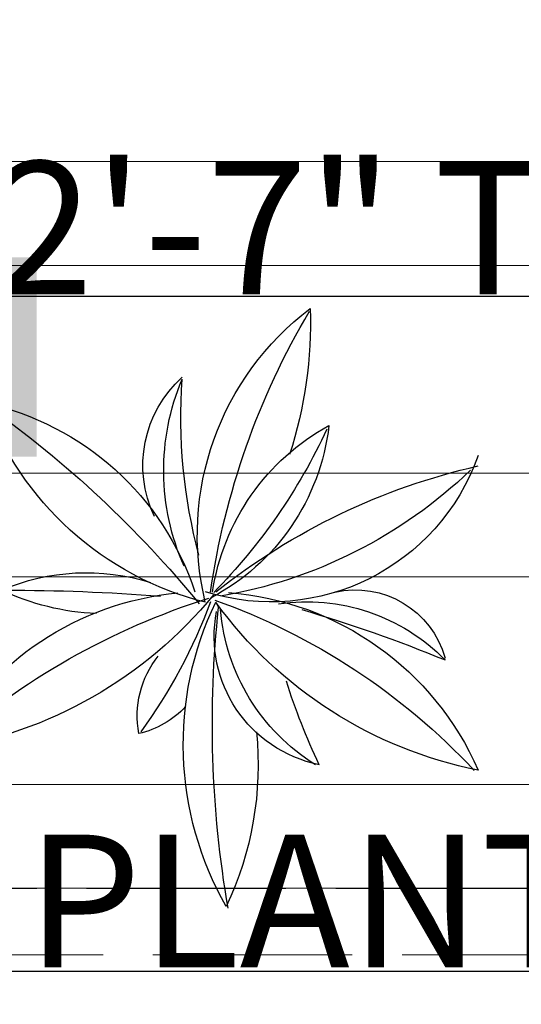
# Model space of a CAD drawing. Units: inches. Extents: x 351 to 1738, y -265 to 286.
# Tile 11 of 38: x 1112 to 1142, y -206 to -147. Entities that reach past the tile are written whole.
import ezdxf

# ---------------------------------------------------------------- set-up
doc = ezdxf.new("R2010")
doc.units = ezdxf.units.IN
doc.header["$MEASUREMENT"] = 0
doc.linetypes.add('ACAD_ISO02W100', pattern=[15, 12, -3])
for name, color, linetype, lineweight in [('A-ANNO-DIMS', 2, 'Continuous', 18), ('A-COLS-PATT', 6, 'Continuous', 13), ('A-FLOR-OVHD', 1, 'ACAD_ISO02W100', 18), ('A-FLOR-PATT', 9, 'Continuous', 9)]:
    doc.layers.add(name, color=color, linetype=linetype, lineweight=lineweight)
for name, color, linetype in [('CAY', 94, 'Continuous'), ('CHITIET', 144, 'Continuous'), ('netmanh', 9, 'Continuous'), ('VATDUNG', 9, 'Continuous')]:
    doc.layers.add(name, color=color, linetype=linetype)
doc.styles.get("Standard").update_dxf_attribs({"font": 'arial.ttf'})
doc.dimstyles.get("Standard").update_dxf_attribs({"dimtxt": 8, "dimasz": 5, "dimexe": 0.18, "dimexo": 0.0625, "dimgap": 0.09, "dimtad": 1, "dimtoh": 1, "dimzin": 0, "dimdsep": 46, "dimlunit": 4, "dimtxsty": 'Standard', "dimcen": 0, "dimclre": 256, "dimadec": 0, "dimazin": 0, "dimtfac": 1, "dimtofl": 0, "dimtmove": 0, "dimatfit": 3, "dimfxl": 1, "dimtolj": 1, "dimtzin": 0, "dimlwe": -1, "dimarcsym": 0})

# ---------------------------------------------------------------- blocks, each defined once
blk = doc.blocks.new('A$C5431134F')
at = {"layer": 'VATDUNG'}
for centre, radius, start, end in [((2160.8, 1662), 1245, 150.2411, 205.809), ((5177, 1582.5), 4150.3, 170.24, 186.1148), ((-65.9, 1738.8), 1267.2, 354.3326, 25.2804), ((1532.8, 1250.1), 499, 101.4267, 190.9877), ((193.1, 3473.3), 2507.8, 289.6318, 316.9416), ((2357.8, 162.2), 1629.1, 101.2486, 143.9899), ((1828.1, 1082.8), 773.2, 121.9055, 175.1859), ((1000.7, 2213.1), 1133.8, 274.4073, 336.4431), ((3715.1, 660.2), 2523.5, 154.6853, 162.4501), ((-246.7, 51.1), 1647.5, 39.15, 81.389), ((1000.7, 2213.1), 1133.8, 208.0484, 264.6491), ((1859.5, 3770.4), 2797.6, 228.5745, 252.3842), ((1101.5, 1552.5), 361.2, 169.1166, 218.9556), ((667.9, 1279.8), 349.9, 42.8374, 76.9786), ((-929.9, 388.9), 2082.1, 20.5138, 36.0242), ((1386.4, 1856.4), 738.5, 261.6389, 315.6255), ((-169.9, 6392.7), 5465.7, 286.3355, 292.415), ((1571.2, 1428.8), 356.3, 257.3557, 344.3532), ((624.5, 223.6), 940.4, 92.4374, 115.2956), ((-65.9, 1738.8), 1267.2, 330.7697, 331.9367), ((1294.4, -49.6), 1206.1, 104.1284, 160.1468), ((-2233.8, 3749.8), 4146.2, 305.4464, 320.7382), ((248.9, 8461.8), 7388, 269.91003, 274.50199), ((2052.7, 864.5), 1083.3, 166.3603, 232.9474), ((1250.8, 281.5), 836.9, 19.4342, 107.4357), ((625, 349.3), 851.8, 6.5073, 62.3609), ((754.1, -691.9), 1814.1, 46.1483, 80.3711), ((-70, 1420), 1084.7, 282.2423, 341.7321), ((546.4, 1826.6), 819.5, 246.7315, 287.3971), ((3885.3, 1488.7), 2894, 188.0959, 210.7226), ((1889.6, 1210.8), 871.9, 188.5552, 241.3289), ((-527.8, -458.7), 2192.5, 24.7599, 44.6473), ((2594.9, 3037.7), 2500, 231.5416, 257.1764), ((1738.9, 617.5), 897.6, 155.9893, 202.84), ((2946.5, 414), 2039.9, 165.0604, 184.0737), ((1214.1, 597.8), 452.1, 154.5276, 228.0163), ((-246.7, 51.1), 1647.5, 358.2222, 17.8583)]:
    blk.add_arc(centre, radius, start, end, dxfattribs=at)
blk = doc.blocks.new('A$C5A8625A6')
at = {"layer": 'CHITIET', "ltscale": 50, "xscale": -0.49, "yscale": 0.49, "zscale": 0.49, "rotation": 180}
blk.add_blockref('A$C5431134F', (0, 1120.2), dxfattribs=at)
blk = doc.blocks.new('A$C18571848')
at = {"layer": 'netmanh', "xscale": 0.5393606399999998, "yscale": 0.5393606399999998, "zscale": 0.5393606399999998}
blk.add_blockref('A$C5A8625A6', (0, 0), dxfattribs=at)
blk = doc.blocks.new('*D36')
at = {"layer": 'A-ANNO-DIMS', "transparency": 16777216}
for p, q in [((1073.569, -199.341), (1073.569, -204.202)), ((1105.198, -199.341), (1105.198, -204.202))]:
    blk.add_line(p, q, dxfattribs=at)
at = {"layer": 'A-ANNO-DIMS', "color": 0, "lineweight": -2, "transparency": 16777216}
for p, q in [((1078.569, -204.022), (1100.198, -204.022)), ((1105.198, -204.022), (1227.071, -204.022))]:
    blk.add_line(p, q, dxfattribs=at)
at = {"layer": 'A-ANNO-DIMS', "color": 0, "transparency": 16777216}
for points in [[(1078.569, -203.189), (1078.569, -204.856), (1073.569, -204.022)], [(1100.198, -203.189), (1100.198, -204.856), (1105.198, -204.022)]]:
    blk.add_solid(points, dxfattribs=at)
at = {"layer": 'Defpoints', "color": 0, "transparency": 16777216}
for p in [(1073.569, -199.278), (1105.198, -199.278), (1105.198, -204.022)]:
    blk.add_point(p, dxfattribs=at)
at = {"layer": 'A-ANNO-DIMS', "color": 0, "transparency": 16777216, "insert": (1168.634, -199.796), "char_height": 8, "attachment_point": 5}
blk.add_mtext('\\A1;PLANT A 2\'-7 1/2" TYP.', dxfattribs=at)
blk = doc.blocks.new('*D37')
at = {"layer": 'A-ANNO-DIMS', "color": 0, "lineweight": -2, "transparency": 16777216}
for p, q in [((1109.942, -168.369), (1109.942, -163.369)), ((1109.942, -163.369), (1158.933, -163.369)), ((1109.942, -194.278), (1109.942, -173.369))]:
    blk.add_line(p, q, dxfattribs=at)
at = {"layer": 'A-ANNO-DIMS', "transparency": 16777216}
for p, q in [((1105.26, -168.369), (1110.122, -168.369)), ((1105.26, -199.278), (1110.122, -199.278))]:
    blk.add_line(p, q, dxfattribs=at)
at = {"layer": 'A-ANNO-DIMS', "color": 0, "transparency": 16777216}
for points in [[(1109.109, -173.369), (1110.775, -173.369), (1109.942, -168.369)], [(1109.109, -194.278), (1110.775, -194.278), (1109.942, -199.278)]]:
    blk.add_solid(points, dxfattribs=at)
at = {"layer": 'Defpoints', "color": 0, "transparency": 16777216}
for p in [(1105.198, -168.369), (1109.942, -168.369), (1105.198, -199.278)]:
    blk.add_point(p, dxfattribs=at)
at = {"layer": 'A-ANNO-DIMS', "color": 0, "transparency": 16777216, "insert": (1134.482, -159.26), "char_height": 8, "attachment_point": 5}
blk.add_mtext('\\A1;2\'-7" TYP.', dxfattribs=at)

msp = doc.modelspace()

# ---------------------------------------------------------------- hatches: boundary and pattern name
at = {"layer": 'A-COLS-PATT'}
h = msp.add_hatch(color=256, dxfattribs=at)
h.dxf.hatch_style = 1
h.paths.add_polyline_path([(1112.704, 237.963), (1103.704, 237.963), (1103.704, 228.963), (1112.704, 228.963)])
h.paths.add_polyline_path([(1115.704, 237.963), (1112.704, 237.963), (1112.704, 228.963), (1115.704, 228.963)])
h.paths.add_polyline_path([(1043.704, 255.963), (1034.704, 255.963), (1034.704, 243.963), (1043.704, 243.963)])
h.paths.add_polyline_path([(1043.704, 210.963), (1034.704, 210.963), (1034.704, 198.963), (1043.704, 198.963)])
h.paths.add_polyline_path([(1043.704, -45.037), (1034.704, -45.037), (1034.704, -57.037), (1043.704, -57.037)])
h.paths.add_polyline_path([(1112.704, -45.037), (1103.704, -45.037), (1103.704, -57.037), (1112.704, -57.037)])
h.paths.add_polyline_path([(1112.704, -161.037), (1103.704, -161.037), (1103.704, -164.037), (1103.704, -173.037), (1112.704, -173.037)])
h.paths.add_polyline_path([(1043.704, -161.037), (1034.704, -161.037), (1034.704, -173.037), (1043.704, -173.037)])
h.paths.add_polyline_path([(1248.549, -164.037), (1236.549, -164.037), (1236.549, -173.037), (1248.549, -173.037)])
h.paths.add_polyline_path([(1248.549, -50), (1236.549, -50), (1236.549, -59), (1248.549, -59)])
h.paths.add_polyline_path([(1248.704, 73.463), (1244.704, 73.463), (1244.704, 64.463), (1248.704, 64.463)])
h.paths.add_polyline_path([(1244.704, 73.463), (1236.704, 73.463), (1236.704, 64.463), (1244.704, 64.463)])
h.paths.add_polyline_path([(1248.704, 237.963), (1236.704, 237.963), (1236.704, 228.963), (1248.704, 228.963)])
h.paths.add_polyline_path([(1392.204, 237.963), (1380.204, 237.963), (1380.204, 228.963), (1392.204, 228.963)])
h.paths.add_polyline_path([(1536.064, 237.963), (1524.064, 237.963), (1524.064, 228.963), (1536.064, 228.963)])
h.paths.add_polyline_path([(1536.064, 73.463), (1524.064, 73.463), (1524.064, 64.463), (1536.064, 64.463)])
h.paths.add_polyline_path([(1384.204, 73.463), (1380.204, 73.463), (1380.204, 64.463), (1384.204, 64.463)])
h.paths.add_polyline_path([(1392.064, 73.463), (1384.204, 73.463), (1384.204, 64.463), (1392.064, 64.463)])
h.paths.add_polyline_path([(1536.064, -53.037), (1524.064, -53.037), (1524.064, -57.037), (1536.064, -57.037)])
h.paths.add_polyline_path([(1536.064, -48.037), (1524.064, -48.037), (1524.064, -53.037), (1536.064, -53.037)])
h.paths.add_polyline_path([(1392.064, -48.037), (1380.064, -48.037), (1380.064, -56.5), (1380.065, -57.037), (1392.064, -57.037)])
h.paths.add_polyline_path([(1536.064, -164.037), (1524.064, -164.037), (1524.064, -173.037), (1536.064, -173.037)])
at = {"layer": 'A-FLOR-PATT', "transparency": 33554559}
h = msp.add_hatch(dxfattribs=at)
h.set_pattern_fill('ANSI37', color=256, scale=200, angle=135)
h.set_pattern_definition([(180, (1112.704, -164.037), (-2e-15, -25), []), (270, (1112.704, -164.037), (25, -5e-15), [])])
h.paths.add_polyline_path([(1380.064, 73.463), (1380.132, 148.463), (1338.064, 148.463), (1290.704, 148.463), (1290.704, 88.463), (1248.704, 88.463), (1248.704, -2.009), (1244.704, -2.009), (1244.704, 142.457), (1160.704, 142.457), (1160.704, 158.963), (1160.704, 170.137), (1160.704, 206.137), (1160.704, 228.963), (1112.704, 228.963), (1112.704, 209.963), (1112.704, 168.963), (1124.704, 168.963), (1124.704, 162.963), (1112.704, 162.963), (1112.704, 64.463), (1112.704, 60.463), (1112.704, 0.463), (1112.704, -48.026), (1146.804, -47.981), (1146.804, -35.691), (1207.804, -35.691), (1207.804, -47.902), (1236.542, -47.864), (1236.544, -50.009), (1248.5, -50.009), (1248.506, -102.915), (1248.512, -150.915), (1248.514, -164.037), (1248.549, -164.037), (1273.017, -164.037), (1273.017, -128.799), (1355.24, -128.799), (1355.24, -164.037), (1384.204, -164.037), (1384.204, -57.037), (1380.064, -57.037), (1380.064, -48.037), (1392.064, -48.037), (1392.064, -53.037), (1406.549, -53.037), (1406.549, -57.037), (1401.204, -57.037), (1401.204, -147.037), (1468.204, -147.037), (1468.204, -138.5), (1472.204, -138.5), (1472.204, -102.5), (1468.204, -102.5), (1468.204, -57.037), (1442.549, -57.037), (1442.549, -53.037), (1463.049, -53.037), (1463.049, -40.747), (1524.049, -40.747), (1524.049, -48.037), (1536.064, -48.037), (1536.064, -53.037), (1557.704, -53.037), (1557.704, 204.963), (1384.204, 204.963), (1384.204, 73.463), (1392.064, 73.463), (1392.064, 64.463), (1384.204, 64.463), (1384.204, -3.5), (1380.204, -3.537), (1380.204, 64.463), (1380.064, 64.463)])
h.paths.add_polyline_path([(1510.714, 86.458, -0.103984), (1511.661, 85.595, 0.470438), (1510.158, 87.614, 0.0961)], flags=16)
h.paths.add_polyline_path([(1510.443, 100.266, 0.009798), (1504.693, 100.48, 0.02879), (1504.6, 99.767, -0.165331), (1505.519, 96.135, -0.143601)], flags=16)
h.paths.add_polyline_path([(1487.201, 85.595, -0.103984), (1488.148, 86.458, 0.0961), (1488.704, 87.614, 0.470438)], flags=0)
h.paths.add_polyline_path([(1495.052, 100.43), (1494.178, 100.43, -0.026463), (1494.262, 99.774, -0.144219)], flags=16)
h.paths.add_polyline_path([(1444.485, 86.458, -0.103984), (1445.433, 85.595, 0.470438), (1443.93, 87.614, 0.0961)], flags=16)
h.paths.add_polyline_path([(1420.972, 85.595, -0.103984), (1421.92, 86.458, 0.0961), (1422.475, 87.614, 0.470438)], flags=16)
h.paths.add_polyline_path([(1428.632, 100.335, 0.001054), (1427.971, 100.309, -0.021524), (1428.033, 99.774, -0.114301)], flags=16)
h.paths.add_polyline_path([(1419.906, 143.708, 0.024979), (1420.222, 157.526), (1421.573, 159.101), (1421.573, 175.369), (1391.393, 175.369), (1391.393, 200.519), (1542.294, 200.519), (1542.294, 175.369), (1512.028, 175.369, 0.019865), (1511.521, 153.838, 0.025134), (1512.758, 118.323, 0.020553), (1512.942, 115.253), (1419.834, 115.253, -0.000414), (1419.843, 124.798), (1413.059, 124.798), (1413.059, 84.437, -0.061853), (1415.831, 80.45, -0.093077), (1420.972, 85.595, -0.267537), (1422.371, 84.732, 0.08511), (1424.052, 84.616, -0.885393), (1424.033, 84.851, -1.125815), (1424.073, 84.366, -0.087987), (1422.371, 84.732, -0.267537), (1422.326, 83.089, -0.370542), (1420.972, 85.595, 0.093077), (1415.831, 80.45, -0.087414), (1417.914, 73.937), (1418.941, 73.937, 0.02725), (1418.913, 76.906, -0.115703), (1421.051, 73.937), (1445.354, 73.937, -0.115703), (1447.492, 76.906, 0.02725), (1447.464, 73.937), (1448.491, 73.937, -0.087414), (1450.574, 80.45, 0.093077), (1445.433, 85.595, -0.370542), (1444.079, 83.089, -0.267537), (1444.034, 84.732, -0.087987), (1442.332, 84.366, -1.125815), (1442.372, 84.851, -2.032736), (1442.364, 84.368, 0.086378), (1444.034, 84.732, -0.267537), (1445.433, 85.595, -0.093077), (1450.574, 80.45, -0.257732), (1466.483, 90.927, -0.47867), (1468.832, 91.907, -0.47867), (1471.18, 90.927, -0.26264), (1483.053, 81.78, -0.071866), (1487.201, 85.595, -0.267537), (1488.6, 84.732, 0.08511), (1490.28, 84.616, -0.885393), (1490.262, 84.851, -1.125815), (1490.301, 84.366, -0.087987), (1488.6, 84.732, -0.267537), (1488.554, 83.089, -0.370542), (1487.201, 85.595, 0.071866), (1483.053, 81.78, -0.132065), (1484.143, 73.937), (1485.169, 73.937, 0.02725), (1485.142, 76.906, -0.115703), (1487.28, 73.937), (1511.582, 73.937, -0.115703), (1513.72, 76.906, 0.02725), (1513.693, 73.937), (1514.719, 73.937, -0.087414), (1516.802, 80.45, 0.093077), (1511.661, 85.595, -0.370542), (1510.308, 83.089, -0.267537), (1510.262, 84.732, -0.087987), (1508.561, 84.366, -1.125815), (1508.601, 84.851, -2.032736), (1508.592, 84.368, 0.086378), (1510.262, 84.732, -0.267537), (1511.661, 85.595, -0.093077), (1516.802, 80.45, -0.061853), (1519.575, 84.437), (1519.575, 73.937), (1413.059, 73.937), (1413.059, 124.798), (1419.843, 124.798, -0.000821)], flags=16)
h.paths.add_polyline_path([(1220.149, 54.133, -0.103984), (1220.869, 53.476, 0.470438), (1219.727, 55.011, 0.0961)], flags=16)
h.paths.add_polyline_path([(1219.944, 64.626, 0.009798), (1215.574, 64.789, 0.02879), (1215.503, 64.247, -0.165331), (1216.201, 61.487, -0.143601)], flags=16)
h.paths.add_polyline_path([(1209.779, 64.449, 0.097446), (1209.339, 64.751), (1208.247, 64.751, 0.12739), (1207.7, 64.326, 0.171586), (1206.95, 61.475, -0.158854), (1207.636, 59.45, 0.015898), (1207.795, 59.218, 0.061546), (1208.598, 59.616, 0.175416), (1208.638, 60.099, -0.284779), (1209.348, 62.472, 0.326216)], flags=16)
h.paths.add_polyline_path([(1169.818, 54.133, -0.103984), (1170.538, 53.476, 0.470438), (1169.396, 55.011, 0.0961)], flags=16)
h.paths.add_polyline_path([(1159.017, 62.472, 0.284764), (1158.307, 60.099, -0.175433), (1158.267, 59.616, 0.39293), (1159.448, 64.449, -0.32623)], flags=16)
h.paths.add_polyline_path([(1156.342, 58.239, -0.178321), (1154.011, 55.31, -0.174736), (1154.722, 55.233, -0.200802), (1156.27, 56.086, 0.12699), (1157.283, 58.991, -0.091205)], flags=16)
h.paths.add_polyline_path([(1156.624, 61.413, 0.157275), (1157.316, 64.247, 0.169622)], flags=16)
h.paths.add_polyline_path([(1152.67, 54.133, -0.0961), (1151.95, 53.476, 0.064076), (1154.465, 54.384, 0.199016)], flags=16)
h.paths.add_polyline_path([(1202.281, 53.476, -0.103984), (1203, 54.133, 0.0961), (1203.423, 55.011, 0.470438)], flags=0)
h.paths.add_polyline_path([(1151.139, 97.64, 0.024979), (1151.379, 108.141), (1152.406, 109.338), (1152.406, 121.701), (1129.47, 121.701), (1129.47, 140.814), (1244.149, 140.814), (1244.149, 121.701), (1221.148, 121.701, 0.019865), (1220.763, 105.338, 0.025134), (1221.703, 78.349, 0.020553), (1221.843, 76.016), (1151.078, 76.016, -0.128743), (1148.786, 65.037, 0.539352), (1150.327, 64.171, -0.027594), (1163.481, 64.751, 0.097695), (1163.04, 64.449, 0.326216), (1163.471, 62.472, -0.284777), (1164.181, 60.099, -0.194757), (1165.846, 61.443, -0.155402), (1165.172, 64.247, -0.166022), (1165.869, 61.475, -0.177014), (1167.852, 62.77, -0.448203), (1169.974, 60.807, -0.393499), (1167.679, 57.86, -0.895548), (1168.438, 54.524, -0.355767), (1166.218, 56.086, -0.066024), (1165.505, 57.539), (1165.251, 56.243, -0.371732), (1164.02, 59.758, -0.373614), (1163.04, 64.449, -0.097695), (1163.481, 64.751, 0.021354), (1153.294, 64.429, -0.134183), (1156.695, 61.368, 0.186873), (1154.636, 62.77, 0.448203), (1152.514, 60.807, 0.403726), (1154.905, 57.846, 0.711219), (1153.334, 55, 0.53154), (1151.95, 53.476, -0.267537), (1153.013, 52.821, 0.08511), (1154.29, 52.732, -0.885393), (1154.276, 52.911, -1.125815), (1154.306, 52.543, -0.087987), (1153.013, 52.821, -0.267537), (1152.978, 51.572, -0.370542), (1151.95, 53.476, 0.093077), (1148.043, 49.566, -0.087414), (1149.626, 44.617), (1150.406, 44.617, 0.02725), (1150.385, 46.873, -0.115703), (1152.01, 44.617), (1170.478, 44.617, -0.115703), (1172.103, 46.873, 0.02725), (1172.082, 44.617), (1172.862, 44.617, -0.087414), (1174.445, 49.566, 0.093077), (1170.538, 53.476, -0.370542), (1169.51, 51.572, -0.267537), (1169.475, 52.821, -0.087987), (1168.182, 52.543, -1.125815), (1168.212, 52.911, -2.032736), (1168.206, 52.544, 0.086378), (1169.475, 52.821, -0.267537), (1170.538, 53.476, -0.093077), (1174.445, 49.566, -0.257732), (1186.536, 57.528, -0.47867), (1188.321, 58.273, -0.47867), (1190.106, 57.528, -0.26264), (1199.128, 50.577, -0.071866), (1202.281, 53.476, -0.267537), (1203.344, 52.821, 0.08511), (1204.621, 52.732, -0.885393), (1204.607, 52.911, -1.125815), (1204.637, 52.543, -0.087987), (1203.344, 52.821, -0.267537), (1203.309, 51.572, -0.370542), (1202.281, 53.476, 0.071866), (1199.128, 50.577, -0.132065), (1199.957, 44.617), (1200.737, 44.617, 0.02725), (1200.716, 46.873, -0.115703), (1202.341, 44.617), (1220.809, 44.617, -0.115703), (1222.434, 46.873, 0.02725), (1222.413, 44.617), (1223.193, 44.617, -0.087414), (1224.776, 49.566, 0.093077), (1220.869, 53.476, -0.370542), (1219.841, 51.572, -0.267537), (1219.806, 52.821, -0.087987), (1218.513, 52.543, -1.125815), (1218.543, 52.911, -2.032736), (1218.537, 52.544, 0.086378), (1219.806, 52.821, -0.267537), (1220.869, 53.476, -0.093077), (1224.776, 49.566, -0.061853), (1226.883, 52.597), (1226.883, 44.617), (1145.936, 44.617), (1145.936, 83.269), (1151.091, 83.269, -0.000821)], flags=16)
h.paths.add_polyline_path([(1218.01, 57.86, -0.895548), (1218.769, 54.524, -0.355767), (1216.549, 56.086, -0.066024), (1215.836, 57.539), (1215.582, 56.243, -0.371732), (1214.351, 59.758, -0.373614), (1213.371, 64.449, 0.326216), (1213.802, 62.472, -0.284777), (1214.512, 60.099, -0.194757), (1216.177, 61.443, -0.179991), (1218.183, 62.77, -0.448203), (1220.305, 60.807, -0.393499)], flags=16)
h.paths.add_polyline_path([(1424.735, 91.363, -0.393499), (1421.715, 95.241, -0.448203), (1424.507, 97.824, -0.179991), (1427.147, 96.077, -0.194757), (1429.338, 94.309, -0.284777), (1430.272, 97.432, 0.326216), (1430.839, 100.034, -0.373614), (1429.55, 93.861, -0.371732), (1427.929, 89.235), (1427.596, 90.941, -0.066024), (1426.657, 89.029, -0.355767), (1423.736, 86.973, -0.895548)], flags=16)
h.paths.add_polyline_path([(1238.033, 131.257, -1), (1227.329, 131.257, -1)], flags=0)
h.paths.add_polyline_path([(1235.357, 131.257, -1), (1230.005, 131.257, -1)], flags=0)
h.paths.add_polyline_path([(1214.039, 54.243, 0.154382), (1214.38, 53.992, 0.358955), (1213.613, 54.016, 0.603948), (1214.379, 53.657, 0.371319), (1213.968, 52.872, 0.187994), (1214.312, 52.809, -0.592455), (1213.953, 52.967, -0.294279), (1214.083, 53.691, -1.300187), (1213.881, 54.134, -0.283762), (1214.469, 53.896, 1.15094)], flags=16)
h.paths.add_polyline_path([(1212.091, 56.286, -0.408434), (1211.337, 56.445, -0.036259), (1211.098, 56.848, -0.236098), (1211.59, 56.63, 0.035345), (1211.835, 56.543, -0.475241), (1212.091, 56.286, -0.475241), (1212.438, 56.182, 0.035345), (1212.631, 56.007, -0.236098), (1213.056, 55.676, -0.036259), (1212.588, 55.697, -0.408434)], flags=16)
h.paths.add_polyline_path([(1211.469, 50.297, 0.296043), (1210.47, 50.527, 0.310883), (1211.931, 50.148, 0.021255)], flags=16)
h.paths.add_polyline_path([(1213.739, 51.818, -0.036259), (1213.271, 51.838, -0.408434), (1212.774, 52.427, -0.094786), (1212.293, 50.703, 1.150474), (1212.911, 50.232, 0.166288), (1213.265, 50.68, -0.025254), (1212.603, 50.13, 1.087932), (1212.471, 49.407, 0.166288), (1213.02, 49.251, -0.016128), (1212.567, 49.563, -0.286859), (1212.217, 49.638, 0.022156), (1212.046, 50.055, -0.64613), (1212.185, 50.498, 0.088412), (1212.732, 52.077, -1.186037), (1213.121, 52.323, 0.035345), (1213.314, 52.148, -0.236098)], flags=16)
h.paths.add_polyline_path([(1212.094, 50.342, -0.048524), (1211.54, 49.605, -1.103834), (1211.397, 48.738, -0.785515), (1211.683, 48.254, -0.392043), (1210.948, 48.525, -0.392819), (1210.561, 47.995, -0.592455), (1210.201, 48.153, -0.294279), (1210.331, 48.877, -0.704172), (1210.316, 49.592, -0.679344), (1210.729, 50.112, 0.563676)], flags=16)
h.paths.add_polyline_path([(1211.274, 49.829, -0.139826), (1210.745, 49.859, -0.217879), (1210.948, 49.509, -0.498572)], flags=0)
h.paths.add_polyline_path([(1433.426, 81.49, -0.181571), (1434.245, 81.788, -0.008067), (1433.726, 82.205, 0.045578), (1432.755, 81.242, 0.179011)], flags=16)
h.paths.add_polyline_path([(1434.146, 81.009, -0.132442), (1433.645, 80.771, 0.259089), (1433.234, 80.471, -0.180211), (1433.392, 80.805, -0.16994), (1432.758, 81.109, 0.032652), (1433.273, 80.474, -0.493363), (1434.046, 80.146, -0.390497)], flags=16)
h.paths.add_polyline_path([(1434.83, 80.047, -0.947538), (1435.294, 79.576, -0.299128), (1434.625, 79.404, -0.270439), (1435.01, 78.591, -0.592455), (1434.537, 78.382, -0.392819), (1434.027, 79.08, -0.392043), (1433.06, 78.723, -0.352042), (1433.003, 79.197, -0.197216), (1433.75, 79.734, -0.71364), (1434.447, 79.939, -0.21479), (1434.819, 80.475, 0.408833), (1435.075, 80.803, -0.226152)], flags=16)
h.paths.add_polyline_path([(1432.67, 81.217, -0.454218), (1431.897, 79.923, -0.414411), (1431.301, 80.035, 0.016129), (1431.897, 80.445, 0.27957), (1432.073, 80.871, -0.289504), (1431.103, 81.321, -0.414411), (1430.978, 81.915, 0.01613), (1431.586, 81.521, 0.341293), (1432.125, 81.583, -0.813186)], flags=16)
h.paths.add_polyline_path([(1429.893, 86.381, -0.947538), (1430.358, 85.91, -0.173106), (1429.984, 85.712, -0.038817), (1431.625, 84.214, -0.0879), (1432.097, 88.549, -0.049768), (1431.254, 88.49, -0.236098), (1431.814, 88.925, 0.035345), (1432.067, 89.155, -0.475241), (1432.524, 89.291, -0.475241), (1432.86, 89.63, 0.035345), (1433.182, 89.744, -0.236098), (1433.83, 90.032, -0.036259), (1433.516, 89.502, -0.408434), (1432.524, 89.291, -0.312424), (1432.106, 88.58, 0.088559), (1431.625, 84.214, -0.408434), (1430.971, 83.439, -0.036259), (1430.355, 83.412, -0.236098), (1430.914, 83.847, 0.035345), (1431.168, 84.078, -0.475241), (1431.625, 84.214, 0.038817), (1429.984, 85.712, -0.321732), (1429.333, 86.048, -0.32743), (1429.883, 86.809, 0.408833), (1430.138, 87.138, -0.226152)], flags=16)
h.paths.add_polyline_path([(1211.206, 58.616, -0.999784), (1211.336, 59.323, -0.614994)], flags=16)
h.paths.add_polyline_path([(1210.288, 49.429, 0.154382), (1210.629, 49.178, 0.358955), (1209.861, 49.202, 0.603948), (1210.627, 48.843, -0.534825), (1210.806, 49.295, 0.748346)], flags=16)
h.paths.add_polyline_path([(1209.589, 51.828, -0.008791), (1209.775, 51.753, 0.112231), (1209.466, 52.019, 1.418851), (1209.014, 51.708, -0.458726), (1208.651, 51.073, -0.592455), (1208.291, 51.232, -0.294279), (1208.421, 51.955, -1.300187), (1208.219, 52.398, -0.226005), (1208.719, 52.257, -0.475519), (1209.158, 52.369, -1.455499), (1209.603, 52.664, 0.421305), (1209.191, 52.262, -0.591212), (1208.979, 51.796, 0.497399), (1209.773, 51.333, 0.649312)], flags=16)
h.paths.add_polyline_path([(1208.029, 52.041, 0.544667), (1208.832, 52.045, 0.220132)], flags=0)
h.paths.add_polyline_path([(1210.438, 51.425, -0.2042), (1210.277, 52.018, 0.270826), (1209.915, 52.897, 0.324115)], flags=0)
h.paths.add_polyline_path([(1209.668, 52.407, -0.60139), (1208.99, 52.221, -0.394916), (1208.248, 52.83, -0.836792), (1208.651, 53.017, -0.338488), (1209.039, 52.571, 0.194138), (1209.191, 52.262, 0.413995), (1209.712, 52.475, 0.51771), (1210.503, 51.416, 0.401922), (1209.493, 50.93, 0.206396), (1209.516, 50.165, -0.319463), (1210.417, 51.418, -0.466635)], flags=16)
h.paths.add_polyline_path([(1206.601, 56.086, -0.355767), (1204.381, 54.524, -0.921198), (1205.236, 57.846, 0.206569), (1207.614, 58.991, -0.12699)], flags=16)
h.paths.add_polyline_path([(1435.487, 82.816, 0.527765), (1436.615, 83.361, 0.50854), (1437.05, 82.433, 0.592455), (1437.524, 82.641, 0.331245), (1436.963, 83.548, 0.387863), (1437.808, 83.626, 0.592954), (1437.618, 84.176, 0.226016), (1436.961, 83.99, 0.318205), (1437.588, 84.854, 0.689374), (1437.05, 84.991, 0.335765), (1436.539, 84.41, -0.156993), (1436.404, 84.065, -0.434611), (1436.961, 83.99, -0.21479), (1437.333, 84.526, 0.408833), (1437.588, 84.854, -0.226152), (1437.343, 84.097, -0.947538), (1437.808, 83.626, -0.299128), (1437.139, 83.455, -0.270439), (1437.524, 82.641, -0.592455), (1437.05, 82.433, -0.392819), (1436.541, 83.13, -0.43966), (1435.475, 82.794, -0.174614), (1435.942, 82.244, -0.206396), (1435.912, 81.237, -0.270826), (1435.125, 82.208, 0.207976), (1434.686, 82.904, -0.196495)], flags=16)
h.paths.add_polyline_path([(1435.386, 84.832, 0.270811), (1434.91, 83.676, -0.204217), (1434.699, 82.895, 0.324115)], flags=0)
h.paths.add_polyline_path([(1435.68, 84.18, -0.217656), (1435.554, 83.304, -0.176705), (1436.236, 83.778, -0.373036)], flags=0)
h.paths.add_polyline_path([(1435.566, 100.034, 0.326216), (1436.133, 97.432, -0.284777), (1437.067, 94.309, -0.194757), (1439.258, 96.077, -0.155402), (1438.371, 99.767, -0.166022), (1439.289, 96.12, -0.177014), (1441.897, 97.824, -0.448203), (1444.69, 95.241, -0.393499), (1441.67, 91.363, -0.895548), (1442.669, 86.973, -0.355767), (1439.748, 89.029, -0.066024), (1438.809, 90.941), (1438.476, 89.235, -0.371732), (1436.855, 93.861, -0.373614)], flags=16)
h.paths.add_polyline_path([(1191.252, 49.507, -0.274022), (1190.658, 48.409, 0.267537), (1191.311, 47.344, 0.370542)], flags=0)
h.paths.add_polyline_path([(1190.301, 49.717, 0.199016), (1188.619, 49.04, 0.064076), (1191.252, 49.507, -0.0961)], flags=0)
h.paths.add_polyline_path([(1189.518, 47.857, 1.125815), (1189.676, 47.523, 2.044605)], flags=0)
h.paths.add_polyline_path([(1464.974, 80.372, 0.274022), (1465.756, 78.927, -0.083013)], flags=0)
h.paths.add_polyline_path([(1464.974, 80.372, 0.370542), (1464.897, 77.525, 0.576324)], flags=0)
h.paths.add_polyline_path([(1464.974, 80.372, -0.470438), (1467.284, 81.372, -0.0961), (1466.226, 80.648, -0.199016), (1468.439, 79.757, -0.064076)], flags=0)
h.paths.add_polyline_path([(1189.511, 56.43, -0.259467), (1188.321, 56.391, -0.259467), (1187.13, 56.43, 0.08511), (1188.193, 55.716, -0.885393), (1188.27, 55.878, -1.196013), (1188.355, 55.442, 0.101459)], flags=0)
h.paths.add_polyline_path([(1188.321, 57.596, 0.078072), (1187.678, 57.24, 0.01555), (1188.321, 57.136, 0.01555), (1188.964, 57.24, 0.078072)], flags=0)
h.paths.add_polyline_path([(1190.164, 55.365, -0.576324), (1190.106, 57.528, -0.198294), (1188.321, 58.319, -0.198294), (1186.536, 57.528, -0.576324), (1186.477, 55.365, -0.370542), (1186.536, 57.528, 0.198294), (1188.321, 58.319, 0.198294), (1190.106, 57.528, -0.370542)], flags=0)
h.paths.add_polyline_path([(1188.372, 55.878, 1.125814), (1188.529, 55.544, 2.044605)], flags=0)
h.paths.add_polyline_path([(1186.341, 49.717, -0.0961), (1185.389, 49.507, 0.064076), (1188.022, 49.04, 0.199016)], flags=0)
h.paths.add_polyline_path([(1185.389, 49.507, -0.267537), (1185.984, 48.409, 0.08511), (1187.046, 47.695, -0.885393), (1187.123, 47.857, -1.125815), (1186.966, 47.523, -0.087987), (1185.984, 48.409, -0.267537), (1185.331, 47.344, -0.370542)], flags=0)
h.paths.add_polyline_path([(1399.441, 187.944, -1), (1413.525, 187.944, -1)], flags=0)
h.paths.add_polyline_path([(1402.962, 187.944, -1), (1410.004, 187.944, -1)], flags=0)
h.paths.add_polyline_path([(1357.663, -72.245), (1377.272, -72.245), (1377.272, -91.854), (1357.663, -91.854)], flags=16)
h.paths.add_polyline_path([(1467.256, 78.201, -1.125815), (1467.049, 77.761, -2.044605)], flags=0)
h.paths.add_polyline_path([(1468.822, 88.714, 0.941125), (1469.106, 88.316, 1.137152), (1468.765, 88.755, 0.890986), (1468.99, 88.245, 0.094828), (1470.398, 89.481, -0.267537), (1471.18, 90.927, -0.028123), (1469.678, 90.547, -0.028774), (1469.948, 90.311, -0.020327), (1468.832, 90.41, -0.020327), (1467.716, 90.311, -0.028774), (1467.986, 90.547, -0.028123), (1466.483, 90.927, -0.267537), (1467.265, 89.481, 0.08511), (1468.663, 88.542, -1.202316)], flags=0)
h.paths.add_polyline_path([(1178.25, 124.523, -0.119929), (1165.65, 124.145, -0.107349), (1159.133, 124.446, -0.102891), (1159.132, 130.465, -0.074897), (1158.993, 137.956, 0.002027), (1167.844, 137.479, -0.07553), (1180.337, 137.666, -0.075861), (1186.502, 137.688, -0.14099), (1186.272, 130.046, -0.095481), (1186.729, 124.748, -0.10603)], flags=0)
h.paths.add_polyline_path([(1469.225, 79.757, -0.199016), (1471.437, 80.648, -0.0961), (1470.379, 81.372, -0.470438), (1472.689, 80.372, -0.370542), (1472.766, 77.525, -0.267537), (1471.907, 78.927, -0.087986), (1470.615, 77.761, -1.125849), (1470.408, 78.201, -2.032736), (1470.642, 77.778, 0.086378), (1471.907, 78.927, -0.267537), (1472.689, 80.372, -0.064076)], flags=0)
h.paths.add_polyline_path([(1430.423, 186.902, -0.074897), (1430.24, 196.758, 0.002027), (1441.887, 196.131, -0.07553), (1458.326, 196.377, -0.075861), (1466.438, 196.406, -0.14099), (1466.136, 186.35, -0.095481), (1466.737, 179.378, -0.10603), (1455.58, 179.082, -0.119929), (1439, 178.585, -0.107349), (1430.425, 178.981, -0.102891)], flags=0)
h.paths.add_polyline_path([(1162.258, 49.939, 0.335765), (1161.87, 49.497, -0.156994), (1161.767, 49.235, -0.434611), (1162.19, 49.178, -0.21479), (1162.473, 49.585, 1.529195)], flags=16)
h.paths.add_polyline_path([(1161.683, 49.021, 0.581518), (1161.268, 49.583, 0.592761)], flags=16)
h.paths.add_polyline_path([(1162.602, 48.058, 0.371319), (1162.192, 48.843, 0.434533), (1162.88, 48.962, 0.185081), (1162.197, 48.926, 1.121837)], flags=16)
h.paths.add_polyline_path([(1161.443, 48.941, -1.307104), (1161.495, 48.571, -0.217752), (1161.136, 48.254, 0.697303), (1161.871, 49.048, 0.121514)], flags=16)
h.paths.add_polyline_path([(1162.531, 49.429, -0.207084), (1162.05, 49.146, -0.99203)], flags=16)
h.paths.add_polyline_path([(1161.304, 49.578, -0.719667), (1161.513, 50.079, -0.130428), (1160.836, 50.168, 0.039593)], flags=0)
h.paths.add_polyline_path([(1162.036, 50.584, -0.008067), (1161.642, 50.9, 0.029367), (1161.35, 50.297, -0.205788)], flags=16)
h.paths.add_polyline_path([(1162.882, 51.392, -0.124733), (1162.763, 51.828, -0.101191), (1162.399, 51.438, -0.153425)], flags=0)
h.paths.add_polyline_path([(1164.235, 51.85, -0.309107), (1164.513, 51.136, -0.627125), (1163.781, 51.603, -0.685909), (1162.777, 51.219, -0.233285), (1163.303, 50.165, -0.270826), (1162.705, 50.903, 0.2042), (1162.381, 51.425, 0.204182), (1162.542, 52.018, -0.270841), (1162.903, 52.897, -0.127261), (1163.219, 52.529, -1.168681), (1163.781, 52.587, -0.329112), (1164.168, 53.017, -0.836792), (1164.571, 52.83, -0.193341), (1164.391, 52.338, -0.947538), (1164.744, 51.981, -0.299128)], flags=16)
h.paths.add_polyline_path([(1163.598, 51.937, -1.262956), (1163.236, 51.831, 0.012575), (1162.971, 51.721, 0.230657), (1163.151, 52.407, -0.164898), (1163.178, 52.661, -0.44932), (1163.628, 52.262, -0.721477), (1164.154, 52.088, -0.849998)], flags=0)
h.paths.add_polyline_path([(1161.613, 58.616, -0.980413), (1161.525, 59.049, -2.908935)], flags=16)
h.paths.add_polyline_path([(1160.252, 49.166, -0.414411), (1159.799, 49.251, 0.016129), (1160.252, 49.563, 0.27957), (1160.386, 49.887, -0.289504), (1159.649, 50.229, -0.414411), (1159.554, 50.68, 0.01613), (1160.015, 50.381, 0.617885), (1160.526, 50.703, -0.094786), (1160.045, 52.427, -0.140444), (1159.682, 52.042, -0.057856), (1159.3, 51.872, 0.544843), (1160.046, 52.419, -0.088122), (1160.404, 55.721, -0.049768), (1159.763, 55.676, -0.236098), (1160.188, 56.007, 0.035345), (1160.381, 56.182, -0.475241), (1160.728, 56.286, -0.475241), (1160.984, 56.543, 0.035345), (1161.229, 56.63, -0.236098), (1161.721, 56.848, -0.036259), (1161.482, 56.445, -0.408434), (1160.728, 56.286, -0.312424), (1160.411, 55.745, 0.088559), (1160.045, 52.427, 0.107081), (1160.634, 50.498, -0.494798), (1160.839, 50.149, -0.454218)], flags=16)
h.paths.add_polyline_path([(1160.666, 49.808, -2.076528), (1160.828, 50.172, 0.019586)], flags=0)
h.paths.add_polyline_path([(1158.439, 53.992, 0.154382), (1158.78, 54.243, 0.748346), (1158.262, 54.109, -0.338225), (1158.492, 53.839, -0.170816), (1159.124, 53.779, 0.495729), (1158.938, 54.134, 0.226016)], flags=16)
h.paths.add_polyline_path([(1160.045, 52.427, 0.038817), (1158.798, 53.565, -0.119818), (1158.574, 53.586, -0.309107), (1158.851, 52.872, -0.187994), (1158.506, 52.809, 0.592455), (1158.866, 52.967, 0.331245), (1158.44, 53.657, 0.201245), (1158.798, 53.565, -0.034023), (1159.901, 52.578, -0.044253), (1159.698, 52.323, -0.475241)], flags=16)
h.paths.add_polyline_path([(1336.926, -95.392), (1336.926, -117.945), (1291.82, -117.945), (1291.82, -95.392)], flags=16)
h.paths.add_polyline_path([(1357.535, -97.244), (1357.726, -96.697, 0.034844)], flags=16)
h.paths.add_polyline_path([(1376.693, -96.478), (1377.301, -96.5, 0.031497), (1375.907, -96.424), (1357.726, -96.424)], flags=16)
h.paths.add_polyline_path([(1379.403, -119.667, 0.026706), (1380.043, -119.439, -0.015299)], flags=16)
h.paths.add_polyline_path([(1357.726, -120.202), (1357.821, -120.202), (1357.821, -120.201)], flags=16)
h.paths.add_polyline_path([(1354.171, -104.592), (1354.469, -98.672, 0.011138)], flags=16)
h.paths.add_polyline_path([(1355.058, -119.136), (1354.578, -118.539, 0.143164)], flags=16)
h.paths.add_polyline_path([(1378.851, -96.821), (1378.85, -96.82), (1378.85, -96.82, -0.04968), (1380.055, -97.191), (1378.85, -96.82, 0.150054), (1375.135, -97.188), (1375.136, -119.44, -0.00997), (1374.747, -116.649), (1357.726, -116.649, 0.169385), (1357.535, -119.382), (1357.535, -119.382), (1357.535, -119.382, 0.034818), (1357.726, -119.928), (1357.726, -119.928), (1357.726, -119.929, -0.034877), (1357.535, -119.382), (1355.507, -119.382), (1355.317, -119.278), (1357.535, -119.382, -0.169394), (1357.726, -116.649, -0.039151), (1374.686, -116.113, -0.002015), (1374.625, -115.546, 0.115322), (1369.915, -115.474, 0.060921), (1369.922, -101.154, 0.115146), (1374.625, -101.079, -0.002016), (1374.686, -100.513, -0.039151), (1357.726, -99.977), (1374.747, -99.977, -0.009963), (1375.135, -97.188), (1375.135, -97.188, -0.150108)], flags=16)
h.paths.add_polyline_path([(1490.963, 91.363, -0.393499), (1487.944, 95.241, -0.448203), (1490.736, 97.824, -0.179991), (1493.376, 96.077, -0.194757), (1495.567, 94.309, -0.284777), (1496.501, 97.432, 0.326216), (1497.068, 100.034, -0.373614), (1495.778, 93.861, -0.371732), (1494.158, 89.235), (1493.824, 90.941, -0.066024), (1492.886, 89.029, -0.355767), (1489.964, 86.973, -0.895548)], flags=16)
h.paths.add_polyline_path([(1354.86, -97.658), (1355.316, -97.348, 0.101911)], flags=16)
h.paths.add_polyline_path([(1497.063, 83.327, 0.176724), (1496.37, 83.785, -0.405139), (1496.016, 83.384, 0.497399), (1497.06, 82.774, 0.649312), (1496.818, 83.426, -0.008791)], flags=16)
h.paths.add_polyline_path([(1496.339, 83.783, 0.592761), (1496.886, 84.522, 0.581518)], flags=16)
h.paths.add_polyline_path([(1495.11, 82.641, 0.592455), (1495.583, 82.433, 0.676915), (1495.805, 83.59, 0.375669)], flags=16)
h.paths.add_polyline_path([(1495.015, 84.176, -0.145057), (1495.301, 84.526, -0.408833), (1495.045, 84.854, 0.220629), (1495.381, 84.152, -0.199594), (1495.851, 83.764, -0.524017), (1494.826, 83.626, -0.592998)], flags=16)
h.paths.add_polyline_path([(1501.655, 81.915, -0.016129), (1501.048, 81.521, -0.392719), (1500.462, 81.37, -0.21067), (1500.607, 81.142, 0.306699)], flags=16)
h.paths.add_polyline_path([(1500.11, 89.291, -0.408434), (1499.118, 89.502, -0.036259), (1498.803, 90.032, -0.236098), (1499.451, 89.744, 0.035345), (1499.774, 89.63, -0.475241), (1500.11, 89.291, -0.475241), (1500.567, 89.155, 0.035345), (1500.82, 88.925, -0.236098), (1501.379, 88.49, -0.036259), (1500.763, 88.516, -0.408434)], flags=16)
h.paths.add_polyline_path([(1498.908, 82.205, -0.051322), (1500.013, 81.134, -0.587931), (1500.234, 81.676, 0.107081), (1501.009, 84.214, -0.03529)], flags=16)
h.paths.add_polyline_path([(1496.93, 83.875, -0.206396), (1497.247, 84.832, -0.270826), (1497.724, 83.676, 0.207976), (1497.944, 82.884, -0.381455)], flags=16)
h.paths.add_polyline_path([(1496.721, 81.237, 0.270812), (1497.509, 82.208, -0.204216), (1497.935, 82.895, 0.324115)], flags=16)
h.paths.add_polyline_path([(1497.529, 80.125, -0.145057), (1497.814, 80.475, -0.703182), (1498.282, 81.178, -0.122925), (1497.977, 81.714, -0.270837), (1499.207, 81.49, 0.207964), (1499.993, 81.248, -0.265145), (1499.278, 80.472, 0.381901), (1498.808, 79.947, -0.305905), (1498.848, 79.519, 0.499482), (1498.574, 79.217, -0.458726), (1498.097, 78.382, -0.592455), (1497.624, 78.591, -0.270439), (1498.009, 79.404, -0.299116), (1497.34, 79.576, -0.593016)], flags=16)
h.paths.add_polyline_path([(1500.736, 79.923, 0.414411), (1501.333, 80.035, -0.321648), (1500.192, 80.765, 0.019886), (1499.976, 81.251, 0.465331)], flags=16)
h.paths.add_polyline_path([(1501.009, 84.214, -0.038817), (1502.649, 85.712, -0.173095), (1502.276, 85.91, -0.593016), (1502.465, 86.46, -0.145057), (1502.751, 86.809, -0.408833), (1502.495, 87.138, 0.220629), (1502.831, 86.436, -0.199594), (1503.301, 86.048, -0.321732), (1502.649, 85.712, 0.038817), (1501.009, 84.214, 0.122449), (1501.412, 83.755, 0.475491), (1501.335, 84.226, 0.055822), (1501.719, 83.847, -0.236098), (1502.278, 83.412, -0.036259), (1501.663, 83.439, -0.408434)], flags=16)
h.paths.add_polyline_path([(1501.794, 100.034, 0.326216), (1502.362, 97.432, -0.284777), (1503.295, 94.309, -0.194757), (1505.486, 96.077, -0.179991), (1508.126, 97.824, -0.448203), (1510.918, 95.241, -0.393499), (1507.899, 91.363, -0.895548), (1508.898, 86.973, -0.355767), (1505.976, 89.029, -0.066024), (1505.038, 90.941), (1504.704, 89.235, -0.371732), (1503.084, 93.861, -0.373614)], flags=16)
h.paths.add_polyline_path([(1146.29, 131.257, -1), (1135.587, 131.257, -1)], flags=0)
h.paths.add_polyline_path([(1143.614, 131.257, -1), (1138.262, 131.257, -1)], flags=0)
h.paths.add_polyline_path([(1524.064, 73.463), (1536.064, 73.463), (1536.064, 64.463), (1524.064, 64.463)], flags=16)
h.paths.add_polyline_path([(1520.162, 187.944, -1), (1534.246, 187.944, -1)], flags=0)
h.paths.add_polyline_path([(1530.725, 187.944), (1527.204, 187.944), (1527.204, 184.423, 0.414214)], flags=0)
h.paths.add_polyline_path([(1278.415, -91.154), (1331.067, -91.154), (1331.067, -80.583), (1278.415, -80.583)], flags=24)
h.paths.add_polyline_path([(1266.655, -79.354), (1354.738, -79.354), (1354.738, -67.817), (1266.655, -67.817)], flags=24)
h.paths.add_polyline_path([(1115.482, 206.184), (1155.098, 206.184), (1155.098, 217.714), (1115.482, 217.714)], flags=24)
h.paths.add_polyline_path([(1161.771, 8.501), (1222.466, 8.501), (1222.466, 19.079), (1161.771, 19.079)], flags=24)
h.paths.add_polyline_path([(1164.656, 18.795), (1210.615, 18.795), (1210.615, 30.324), (1164.656, 30.324)], flags=24)
h.paths.add_polyline_path([(1368.147, -32.882), (1379.362, -32.882), (1379.362, -21.733), (1368.147, -21.733)], flags=24)
h.paths.add_polyline_path([(1244.842, -31.012), (1256.057, -31.012), (1256.057, -19.863), (1244.842, -19.863)], flags=24)
h.paths.add_polyline_path([(1114.589, 195.739), (1156.517, 195.739), (1156.517, 206.31), (1114.589, 206.31)], flags=24)
h.paths.add_polyline_path([(1436.398, 37.632), (1505.131, 37.632), (1505.131, 48.203), (1436.398, 48.203)], flags=24)
h.paths.add_polyline_path([(1435.991, 47.919), (1507.906, 47.919), (1507.906, 59.456), (1435.991, 59.456)], flags=24)
h.paths.add_polyline_path([(1415.107, -124.896), (1457.038, -124.896), (1457.038, -114.318), (1415.107, -114.318)], flags=24)
h.paths.add_polyline_path([(1417.992, -114.602), (1457.609, -114.602), (1457.609, -103.073), (1417.992, -103.073)], flags=24)
h = msp.add_hatch(dxfattribs=at)
h.set_pattern_fill('ANSI32', color=256, scale=50, angle=135)
h.set_pattern_definition([(180, (1038.704, -199.037), (-2e-15, -18.75), []), (180, (1032.454, -192.787), (-2e-15, -18.75), [])])
h.paths.add_polyline_path([(1248.506, -102.915), (1236.559, -102.916), (1236.553, -56.864), (1112.704, -57.026), (1112.704, -57.037), (1103.704, -57.037), (1103.704, -45.037), (1103.704, 98.963), (1076.434, 98.963), (1076.549, -81.037), (1071.549, -81.037), (1043.704, -81.037), (1038.704, -81.037), (1038.704, -161.037), (1043.704, -161.037), (1043.704, -173.037), (1038.704, -173.037), (1038.704, -199.037), (1562.704, -199.037), (1562.704, -173.037), (1236.549, -173.037), (1236.549, -164.037), (1236.693, -164.037), (1236.676, -150.916), (1248.512, -150.915)])
h.paths.add_polyline_path([(1236.133, -134.078), (1247.348, -134.078), (1247.348, -122.929), (1236.133, -122.929)], flags=24)
h.paths.add_polyline_path([(1308.144, -185.548), (1321.66, -185.548), (1321.66, -174.4), (1308.144, -174.4)], flags=24)
h.paths.add_polyline_path([(1121.632, -122.88), (1179.647, -122.88), (1179.647, -112.309), (1121.632, -112.309)], flags=24)
h.paths.add_polyline_path([(1124.515, -112.593), (1177.986, -112.593), (1177.986, -101.056), (1124.515, -101.056)], flags=24)
h.paths.add_polyline_path([(1091.374, 23.58), (1104.89, 23.58), (1104.89, 34.728), (1091.374, 34.728)], flags=24)

# ---------------------------------------------------------------- linework, layer by layer
at = {"layer": 'A-FLOR-OVHD'}
for p, q in [((1562.704, -199.037), (1038.704, -199.037)), ((1566.704, -203.037), (1034.704, -203.037))]:
    msp.add_line(p, q, dxfattribs=at)

# ---------------------------------------------------------------- block references
at = {"layer": 'CAY', "xscale": 0.0597507335965459, "yscale": 0.0597507335965459, "zscale": 0.0597507335965459}
msp.add_blockref('A$C18571848', (1107.065, -200.223), dxfattribs=at)

# ---------------------------------------------------------------- dimensions: what is measured, and where the dimension line sits
at = {"layer": 'A-ANNO-DIMS'}
dim = msp.add_linear_dim(base=(1109.942, -168.369), p1=(1105.198, -199.278), p2=(1105.198, -168.369), angle=90, text='<> TYP.', dimstyle='Standard', override={"dimdec": 1, "dimlfac": 1, "dimrnd": 0, "dimzin": 1, "dimdsep": 46, "dimlunit": 4, "dimfrac": 2}, dxfattribs=at)
dim.commit()
dim.dimension.update_dxf_attribs({"geometry": '*D37', "text_midpoint": (1134.482, -159.26)})
dim = msp.add_linear_dim(base=(1105.198, -204.022), p1=(1073.569, -199.278), p2=(1105.198, -199.278), text='PLANT A <> TYP.', dimstyle='Standard', override={"dimdec": 1, "dimlfac": 1, "dimrnd": 0, "dimzin": 1, "dimdsep": 46, "dimlunit": 4, "dimfrac": 2}, dxfattribs=at)
dim.commit()
dim.dimension.update_dxf_attribs({"geometry": '*D36', "text_midpoint": (1168.634, -199.796)})

doc.saveas('drawing.dxf')
